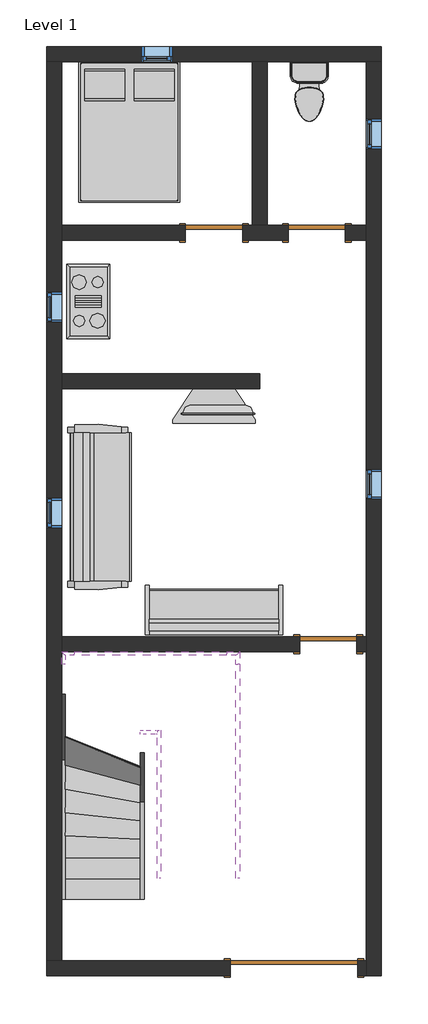
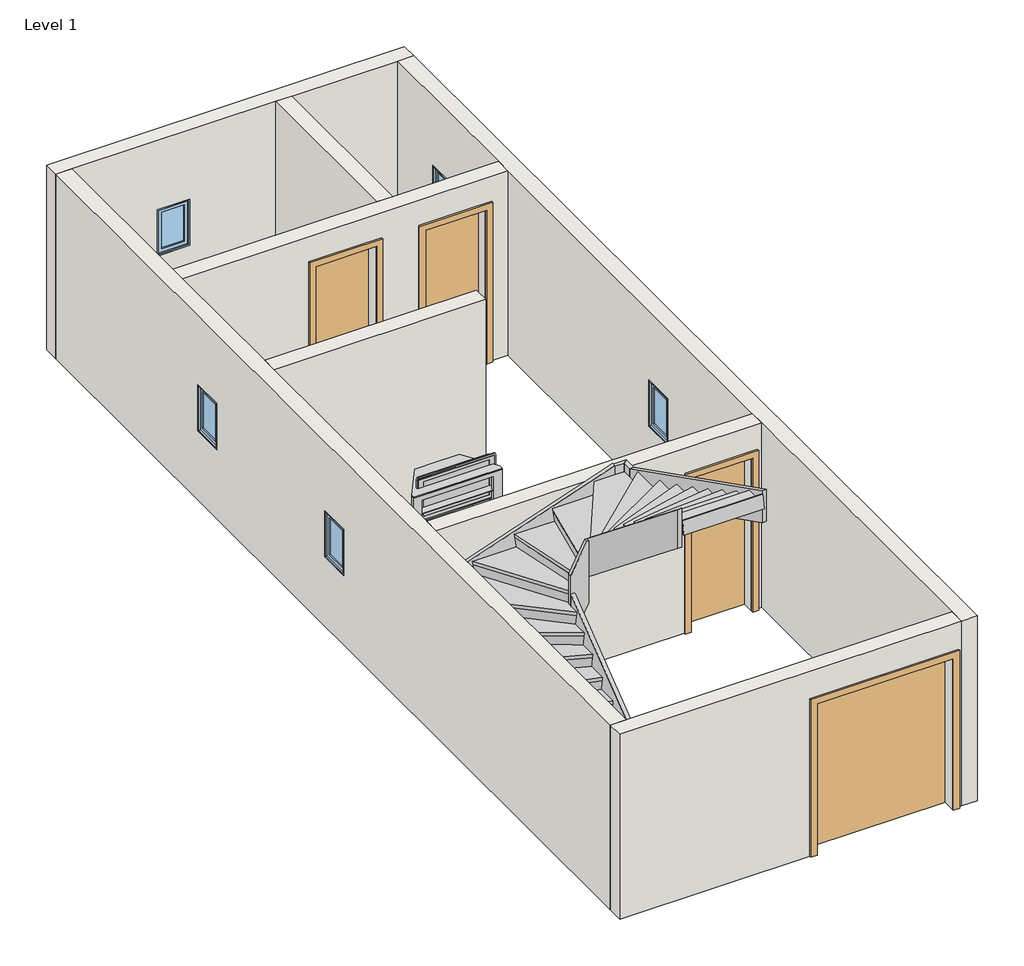
# One storey, incomplete: 10 members, 8 walls, 5 furniture elements, 5 windows, 4 doors, 1 flow terminal, 1 proxy, 1 stair flight.
"""IFC4 building model written with IfcOpenShell, lengths in millimetres."""

from ifc_helpers import new_model, si_unit, frame, origin, origin_with_axes, place, context, project, spatial, polyline, outline, extrude, faceted_brep, transform, mapped, element, save
from components import m_cook_top_4_unit_0915_x_500mm_0d6b06ed, m_door_double_flush_panel_double_acting_1700_x_2000mm_0a6d9c7f, m_single_flush_0762_x_2032mm_0c256fab, m_toilet_domestic_3d_m_toilet_domestic_3d_5cb52bd4, m_toilet_domestic_3d_m_toilet_domestic_3d_183bbd19, furniture_40ec15d9, furniture_0940mm_4831bac8, m_bed_box_1346_x_1880mm_double_b32eb57e, m_sofa_1830mm_f9e8a66b, m_sofa_pensi_2134mm_91f3548c, stair_flight_50mm_tread_25mm_nosing_13mm_riser_90fcb94b, m_fixed_0406_x_0610mm_8205b201

model = new_model("IFC4")

# Units and contexts
model_context = context("Model", 3, world=origin())
ifc_project = project(units=[si_unit("LENGTHUNIT", "METRE", prefix="MILLI")], contexts=[model_context])

# Site, building, storey
site = spatial("IfcSite", under=ifc_project)
building = spatial("IfcBuilding", under=site)
storey = spatial("IfcBuildingStorey", under=building, Name="Level 1", Elevation=0.0)

# Proxy
placement = place(None, origin())
m_cook_top_4_unit_0915_x_500mm_shape = m_cook_top_4_unit_0915_x_500mm_0d6b06ed(model_context)
element("IfcBuildingElementProxy", 1, Name="M_Cook Top-4 Unit : 0915 x 500mm", ObjectType="M_Cook Top-4 Unit : 0915 x 500mm", at=placement, inside=storey, context=model_context, shape_type="MappedRepresentation", body=[
    mapped(m_cook_top_4_unit_0915_x_500mm_shape, transform((-8350.9652156, 7282.492595, 0.0), x_axis=(0.0, 1.0000000000000002, 0.0), y_axis=(-1.0000000000000002, 0.0, 0.0), z_axis=(0.0, 0.0, 1.0))),
])

# Doors
m_door_double_flush_panel_double_acting_1700_x_2000mm_shape = m_door_double_flush_panel_double_acting_1700_x_2000mm_0a6d9c7f(model_context)
element("IfcDoor", 2, ObjectType="M_Door-Double-Flush_Panel-Double-Acting : 1700 x 2000mm", at=placement, inside=storey, context=model_context, shape_type="MappedRepresentation", body=[
    mapped(m_door_double_flush_panel_double_acting_1700_x_2000mm_shape, transform((-5607.7652156, -1609.107405, 0.0), x_axis=(1.0, 0.0, 0.0), y_axis=(0.0, 1.0, 0.0), z_axis=(0.0, 0.0, 1.0))),
])
m_single_flush_0762_x_2032mm_shape = m_single_flush_0762_x_2032mm_0c256fab(model_context)
element("IfcDoor", 3, ObjectType="M_Single-Flush : 0762 x 2032mm", at=placement, inside=storey, context=model_context, shape_type="MappedRepresentation", body=[
    mapped(m_single_flush_0762_x_2032mm_shape, transform((-6674.5652156, 8196.892595, 0.0), x_axis=(1.0, 0.0, 0.0), y_axis=(0.0, 1.0, 0.0), z_axis=(0.0, 0.0, 1.0))),
])
element("IfcDoor", 4, ObjectType="M_Single-Flush : 0762 x 2032mm", at=placement, inside=storey, context=model_context, shape_type="MappedRepresentation", body=[
    mapped(m_single_flush_0762_x_2032mm_shape, transform((-5302.9652156, 8196.892595, 0.0), x_axis=(1.0, 0.0, 0.0), y_axis=(0.0, 1.0, 0.0), z_axis=(0.0, 0.0, 1.0))),
])
element("IfcDoor", 5, ObjectType="M_Single-Flush : 0762 x 2032mm", at=placement, inside=storey, context=model_context, shape_type="MappedRepresentation", body=[
    mapped(m_single_flush_0762_x_2032mm_shape, transform((-5150.5652156, 2710.492595, 0.0), x_axis=(1.0, 0.0, 0.0), y_axis=(0.0, 1.0, 0.0), z_axis=(0.0, 0.0, 1.0))),
])

# Flow terminal
m_toilet_domestic_3d_m_toilet_domestic_3d_shape = m_toilet_domestic_3d_m_toilet_domestic_3d_5cb52bd4(model_context)
m_toilet_domestic_3d_m_toilet_domestic_3d_2_shape = m_toilet_domestic_3d_m_toilet_domestic_3d_183bbd19(model_context)
element("IfcFlowTerminal", 6, ObjectType="M_Toilet-Domestic-3D : M_Toilet-Domestic-3D", at=placement, inside=storey, context=model_context, shape_type="MappedRepresentation", body=[
    mapped(m_toilet_domestic_3d_m_toilet_domestic_3d_shape, transform((-5403.961243, 9988.1965677, 0.0), x_axis=(1.0, 0.0, 0.0), y_axis=(0.0, 1.0, 0.0), z_axis=(0.0, 0.0, 1.0))),
    mapped(m_toilet_domestic_3d_m_toilet_domestic_3d_2_shape, transform((-5403.961243, 9988.1965677, 0.0), x_axis=(1.0, 0.0, 0.0), y_axis=(0.0, 1.0, 0.0), z_axis=(0.0, 0.0, 1.0))),
])

# Furniture
furniture_shape = furniture_40ec15d9(model_context)
element("IfcFurniture", 7, at=placement, inside=storey, context=model_context, shape_type="MappedRepresentation", body=[
    mapped(furniture_shape, transform((-6799.7532177, 6115.692595, 0.0), x_axis=(1.0, 0.0, 0.0), y_axis=(0.0, 1.0, 0.0), z_axis=(0.0, 0.0, 1.0))),
])
furniture_0940mm_shape = furniture_0940mm_4831bac8(model_context)
element("IfcFurniture", 8, ObjectType="0940mm", at=placement, inside=storey, context=model_context, shape_type="MappedRepresentation", body=[
    mapped(furniture_0940mm_shape, transform((-6619.8207015, 5844.2185016, 0.0), x_axis=(1.0, 0.0, 0.0), y_axis=(0.0, 1.0, 0.0), z_axis=(0.0, 0.0, 1.0))),
])
m_bed_box_1346_x_1880mm_double_shape = m_bed_box_1346_x_1880mm_double_b32eb57e(model_context)
element("IfcFurniture", 9, ObjectType="M_Bed-Box : 1346 x 1880mm - Double", at=placement, inside=storey, context=model_context, shape_type="MappedRepresentation", body=[
    mapped(m_bed_box_1346_x_1880mm_double_shape, transform((-8143.9176746, 9777.3221032, 0.0), x_axis=(1.0, 0.0, 0.0), y_axis=(0.0, 1.0, 0.0), z_axis=(0.0, 0.0, 1.0))),
])
m_sofa_1830mm_shape = m_sofa_1830mm_f9e8a66b(model_context)
element("IfcFurniture", 10, ObjectType="M_Sofa : 1830mm", at=placement, inside=storey, context=model_context, shape_type="MappedRepresentation", body=[
    mapped(m_sofa_1830mm_shape, transform((-6604.1947238, 3313.8466934, 0.0), x_axis=(-1.0000000000000004, 0.0, 0.0), y_axis=(0.0, -1.0000000000000004, 0.0), z_axis=(0.0, 0.0, 1.0))),
])
m_sofa_pensi_2134mm_shape = m_sofa_pensi_2134mm_91f3548c(model_context)
element("IfcFurniture", 11, ObjectType="M_Sofa-Pensi : 2134mm", at=placement, inside=storey, context=model_context, shape_type="MappedRepresentation", body=[
    mapped(m_sofa_pensi_2134mm_shape, transform((-7921.4553795, 4260.686345, 0.0), x_axis=(0.0, 1.0, 0.0), y_axis=(-1.0, 0.0, 0.0), z_axis=(0.0, 0.0, 1.0))),
])

# Members
element("IfcMember", 12, ObjectType="Stringer - 50mm Width", at=placement, inside=storey, context=model_context, shape_type="SweptSolid", body=[
    extrude(outline(polyline([(-689.3306191, 0.0), (-689.3306191, 237.7763786), (2445.6423401, 1858.1790604), (2445.6423401, 1407.9055029), (-278.2149643, 0.0), (-689.3306191, 0.0)])), frame((-8708.1652156, 0.0, 0.0), z_axis=(1.0, 0.0, 0.0), x_axis=(0.0, 1.0, 0.0)), (0.0, 0.0, 1.0), 50.0),
])
element("IfcMember", 13, ObjectType="Stringer - 50mm Width", at=placement, inside=storey, context=model_context, shape_type="SweptSolid", body=[
    extrude(outline(polyline([(-8658.1652156, 2445.6423401), (-8708.1652156, 2445.6423401), (-8708.1652156, 2610.492595), (-8658.1652156, 2560.492595), (-8658.1652156, 2445.6423401)])), frame((0.0, 0.0, 1407.9055029), z_axis=(0.0, 0.0, 1.0), x_axis=(1.0, 0.0, 0.0)), (0.0, 0.0, 1.0), 450.2735574),
])
element("IfcMember", 14, ObjectType="Stringer - 50mm Width", at=placement, inside=storey, context=model_context, shape_type="SweptSolid", body=[
    extrude(outline(polyline([(-8658.1652156, 2560.492595), (-8708.1652156, 2610.492595), (-8536.9547066, 2610.492595), (-8536.9547066, 2560.492595), (-8658.1652156, 2560.492595)])), frame((0.0, 0.0, 1407.9055029), z_axis=(0.0, 0.0, 1.0), x_axis=(1.0, 0.0, 0.0)), (0.0, 0.0, 1.0), 450.2735574),
])
element("IfcMember", 15, ObjectType="Stringer - 50mm Width", at=placement, inside=storey, context=model_context, shape_type="SweptSolid", body=[
    extrude(outline(polyline([(1858.1790604, -8536.9547066), (1407.9055029, -8536.9547066), (2103.5576768, -6502.8954819), (2553.8312343, -6502.8954819), (1858.1790604, -8536.9547066)])), frame((0.0, 2560.492595, 0.0), z_axis=(0.0, 1.0, 0.0), x_axis=(0.0, 0.0, 1.0)), (0.0, 0.0, 1.0), 50.0),
])
element("IfcMember", 16, ObjectType="Stringer - 50mm Width", at=placement, inside=storey, context=model_context, shape_type="SweptSolid", body=[
    extrude(outline(polyline([(-6502.8954819, 2560.492595), (-6502.8954819, 2610.492595), (-6333.1136531, 2610.492595), (-6383.1136531, 2560.492595), (-6502.8954819, 2560.492595)])), frame((0.0, 0.0, 2121.8553305), z_axis=(0.0, 0.0, 1.0), x_axis=(1.0, 0.0, 0.0)), (0.0, 0.0, 1.0), 422.7463197),
])
element("IfcMember", 17, ObjectType="Stringer - 50mm Width", at=placement, inside=storey, context=model_context, shape_type="SweptSolid", body=[
    extrude(outline(polyline([(-6383.1136531, 2560.492595), (-6333.1136531, 2610.492595), (-6333.1136531, 2442.5214684), (-6383.1136531, 2442.5214684), (-6383.1136531, 2560.492595)])), frame((0.0, 0.0, 2121.8553305), z_axis=(0.0, 0.0, 1.0), x_axis=(1.0, 0.0, 0.0)), (0.0, 0.0, 1.0), 422.7463197),
])
element("IfcMember", 18, ObjectType="Stringer - 50mm Width", at=placement, inside=storey, context=model_context, shape_type="SweptSolid", body=[
    extrude(outline(polyline([(2442.5214684, 2544.6016503), (2442.5214684, 2121.8553305), (-414.3306191, 3565.1327467), (-414.3306191, 3987.8790664), (2442.5214684, 2544.6016503)])), frame((-6383.1136531, 0.0, 0.0), z_axis=(1.0, 0.0, 0.0), x_axis=(0.0, 1.0, 0.0)), (0.0, 0.0, 1.0), 50.0),
])
element("IfcMember", 19, ObjectType="Stringer - 50mm Width", at=placement, inside=storey, context=model_context, shape_type="SweptSolid", body=[
    extrude(outline(polyline([(-689.3306191, 0.0), (-689.3306191, 189.4989591), (1510.4668138, 1898.4837123), (1510.4668138, 1391.9587893), (-281.2562345, 0.0), (-689.3306191, 0.0)])), frame((-7658.1394344, 0.0, 0.0), z_axis=(1.0, 0.0, 0.0), x_axis=(0.0, 1.0, 0.0)), (0.0, 0.0, 1.0), 50.0),
])
element("IfcMember", 20, ObjectType="Stringer - 50mm Width", at=placement, inside=storey, context=model_context, shape_type="SweptSolid", body=[
    extrude(outline(polyline([(2137.8523026, -7658.1394344), (1430.8029285, -7658.1394344), (1430.8029285, -7575.3363491), (1703.8772172, -7433.1394344), (2523.9527077, -7433.1394344), (2523.9527077, -7457.0868686), (2137.8523026, -7658.1394344)])), frame((0.0, 1510.4668138, 0.0), z_axis=(0.0, 1.0, 0.0), x_axis=(0.0, 0.0, 1.0)), (0.0, 0.0, 1.0), 50.0),
])
element("IfcMember", 21, ObjectType="Stringer - 50mm Width", at=placement, inside=storey, context=model_context, shape_type="SweptSolid", body=[
    extrude(outline(polyline([(1560.4668138, 2523.9527077), (1560.4668138, 2011.6830523), (-414.3306191, 3591.6768139), (-414.3306191, 4103.9464694), (1560.4668138, 2523.9527077)])), frame((-7433.1394344, 0.0, 0.0), z_axis=(1.0, 0.0, 0.0), x_axis=(0.0, 1.0, 0.0)), (0.0, 0.0, 1.0), 50.0),
])

# Stair flight
stair_flight_50mm_tread_25mm_nosing_13mm_riser_shape = stair_flight_50mm_tread_25mm_nosing_13mm_riser_90fcb94b(model_context)
element("IfcStairFlight", 22, ObjectType="50mm Tread 25mm Nosing 13mm Riser", at=placement, inside=storey, context=model_context, shape_type="MappedRepresentation", body=[
    mapped(stair_flight_50mm_tread_25mm_nosing_13mm_riser_shape, transform((0.0, 0.0, 0.0), x_axis=(1.0, 0.0, 0.0), y_axis=(0.0, 1.0, 0.0), z_axis=(0.0, 0.0, 1.0))),
])

# Walls
element("IfcWall", 23, ObjectType="Generic - 200mm", at=placement, inside=storey, context=model_context, shape_type="Brep", body=[
    faceted_brep([(-8908.1652156, 10482.892595, 0.0), (-8708.1652156, 10482.892595, 0.0), (-6164.9652156, 10482.892595, 0.0), (-5964.9652156, 10482.892595, 0.0), (-4640.9652156, 10482.892595, 0.0), (-4440.9652156, 10482.892595, 0.0), (-4440.9652156, 10482.892595, 2438.4), (-4640.9652156, 10482.892595, 2438.4), (-5964.9652156, 10482.892595, 2438.4), (-6164.9652156, 10482.892595, 2438.4), (-8708.1652156, 10482.892595, 2438.4), (-8908.1652156, 10482.892595, 2438.4), (-7233.5652156, 10482.892595, 915.0), (-7639.5652156, 10482.892595, 915.0), (-7639.5652156, 10482.892595, 1525.0), (-7233.5652156, 10482.892595, 1525.0), (-8908.1652156, 10682.892595, 0.0), (-8908.1652156, 10682.892595, 2438.4), (-4440.9652156, 10682.892595, 2438.4), (-4440.9652156, 10682.892595, 0.0), (-7233.5652156, 10682.892595, 915.0), (-7233.5652156, 10682.892595, 1525.0), (-7639.5652156, 10682.892595, 1525.0), (-7639.5652156, 10682.892595, 915.0)], [[[0, 1, 2, 3, 4, 5, 6, 7, 8, 9, 10, 11], [12, 13, 14, 15]], [[16, 17, 18, 19], [20, 21, 22, 23]], [[5, 4, 3, 2, 1, 0, 16, 19]], [[11, 10, 9, 8, 7, 6, 18, 17]], [[6, 5, 19, 18]], [[0, 11, 17, 16]], [[21, 20, 12, 15]], [[22, 21, 15, 14]], [[23, 22, 14, 13]], [[20, 23, 13, 12]]]),
])
element("IfcWall", 24, ObjectType="Generic - 200mm", at=placement, inside=storey, context=model_context, shape_type="Brep", body=[
    faceted_brep([(-4640.9652156, 10482.892595, 0.0), (-4640.9652156, 8296.892595, 0.0), (-4640.9652156, 8096.892595, 0.0), (-4640.9652156, 2810.492595, 0.0), (-4640.9652156, 2610.492595, 0.0), (-4640.9652156, -1509.107405, 0.0), (-4640.9652156, -1709.107405, 0.0), (-4640.9652156, -1709.107405, 2438.4), (-4640.9652156, -1509.107405, 2438.4), (-4640.9652156, 2610.492595, 2438.4), (-4640.9652156, 2810.492595, 2438.4), (-4640.9652156, 8096.892595, 2438.4), (-4640.9652156, 8296.892595, 2438.4), (-4640.9652156, 10482.892595, 2438.4), (-4640.9652156, 4641.092595, 915.0), (-4640.9652156, 5047.092595, 915.0), (-4640.9652156, 5047.092595, 1525.0), (-4640.9652156, 4641.092595, 1525.0), (-4640.9652156, 9313.092595, 915.0), (-4640.9652156, 9719.092595, 915.0), (-4640.9652156, 9719.092595, 1525.0), (-4640.9652156, 9313.092595, 1525.0), (-4440.9652156, 10482.892595, 0.0), (-4440.9652156, 10482.892595, 2438.4), (-4440.9652156, -1709.107405, 2438.4), (-4440.9652156, -1709.107405, 0.0), (-4440.9652156, 4641.092595, 915.0), (-4440.9652156, 4641.092595, 1525.0), (-4440.9652156, 5047.092595, 1525.0), (-4440.9652156, 5047.092595, 915.0), (-4440.9652156, 9313.092595, 915.0), (-4440.9652156, 9313.092595, 1525.0), (-4440.9652156, 9719.092595, 1525.0), (-4440.9652156, 9719.092595, 915.0)], [[[0, 1, 2, 3, 4, 5, 6, 7, 8, 9, 10, 11, 12, 13], [14, 15, 16, 17], [18, 19, 20, 21]], [[22, 23, 24, 25], [26, 27, 28, 29], [30, 31, 32, 33]], [[6, 5, 4, 3, 2, 1, 0, 22, 25]], [[13, 12, 11, 10, 9, 8, 7, 24, 23]], [[0, 13, 23, 22]], [[7, 6, 25, 24]], [[27, 26, 14, 17]], [[28, 27, 17, 16]], [[29, 28, 16, 15]], [[26, 29, 15, 14]], [[31, 30, 18, 21]], [[32, 31, 21, 20]], [[33, 32, 20, 19]], [[30, 33, 19, 18]]]),
])
element("IfcWall", 25, ObjectType="Generic - 200mm", at=placement, inside=storey, context=model_context, shape_type="Brep", body=[
    faceted_brep([(-8908.1652156, -1509.107405, 2438.4), (-8708.1652156, -1509.107405, 2438.4), (-4640.9652156, -1509.107405, 2438.4), (-4640.9652156, -1509.107405, 0.0), (-4757.7652156, -1509.107405, 0.0), (-4757.7652156, -1509.107405, 2000.0), (-6457.7652156, -1509.107405, 2000.0), (-6457.7652156, -1509.107405, 0.0), (-8708.1652156, -1509.107405, 0.0), (-8908.1652156, -1509.107405, 0.0), (-4640.9652156, -1709.107405, 2438.4), (-8908.1652156, -1709.107405, 2438.4), (-8908.1652156, -1709.107405, 0.0), (-6457.7652156, -1709.107405, 0.0), (-6457.7652156, -1709.107405, 2000.0), (-4757.7652156, -1709.107405, 2000.0), (-4757.7652156, -1709.107405, 0.0), (-4640.9652156, -1709.107405, 0.0)], [[[0, 1, 2, 3, 4, 5, 6, 7, 8, 9]], [[10, 11, 12, 13, 14, 15, 16, 17]], [[3, 17, 16, 4]], [[12, 9, 8, 7, 13]], [[2, 1, 0, 11, 10]], [[3, 2, 10, 17]], [[0, 9, 12, 11]], [[15, 5, 4, 16]], [[5, 15, 14, 6]], [[6, 14, 13, 7]]]),
])
element("IfcWall", 26, ObjectType="Generic - 200mm", at=placement, inside=storey, context=model_context, shape_type="Brep", body=[
    faceted_brep([(-8708.1652156, -1509.107405, 0.0), (-8708.1652156, 2610.492595, 0.0), (-8708.1652156, 2810.492595, 0.0), (-8708.1652156, 6115.692595, 0.0), (-8708.1652156, 6315.692595, 0.0), (-8708.1652156, 8096.892595, 0.0), (-8708.1652156, 8296.892595, 0.0), (-8708.1652156, 10482.892595, 0.0), (-8708.1652156, 10482.892595, 2438.4), (-8708.1652156, 8296.892595, 2438.4), (-8708.1652156, 8096.892595, 2438.4), (-8708.1652156, 6315.692595, 2438.4), (-8708.1652156, 6115.692595, 2438.4), (-8708.1652156, 2810.492595, 2438.4), (-8708.1652156, 2610.492595, 2438.4), (-8708.1652156, -1509.107405, 2438.4), (-8708.1652156, 7003.292595, 915.0), (-8708.1652156, 7003.292595, 1525.0), (-8708.1652156, 7409.292595, 1525.0), (-8708.1652156, 7409.292595, 915.0), (-8708.1652156, 4260.092595, 915.0), (-8708.1652156, 4260.092595, 1525.0), (-8708.1652156, 4666.092595, 1525.0), (-8708.1652156, 4666.092595, 915.0), (-8908.1652156, -1509.107405, 0.0), (-8908.1652156, -1509.107405, 2438.4), (-8908.1652156, 10482.892595, 2438.4), (-8908.1652156, 10482.892595, 0.0), (-8908.1652156, 7003.292595, 915.0), (-8908.1652156, 7409.292595, 915.0), (-8908.1652156, 7409.292595, 1525.0), (-8908.1652156, 7003.292595, 1525.0), (-8908.1652156, 4260.092595, 915.0), (-8908.1652156, 4666.092595, 915.0), (-8908.1652156, 4666.092595, 1525.0), (-8908.1652156, 4260.092595, 1525.0)], [[[0, 1, 2, 3, 4, 5, 6, 7, 8, 9, 10, 11, 12, 13, 14, 15], [16, 17, 18, 19], [20, 21, 22, 23]], [[24, 25, 26, 27], [28, 29, 30, 31], [32, 33, 34, 35]], [[7, 6, 5, 4, 3, 2, 1, 0, 24, 27]], [[15, 14, 13, 12, 11, 10, 9, 8, 26, 25]], [[8, 7, 27, 26]], [[0, 15, 25, 24]], [[17, 16, 28, 31]], [[18, 17, 31, 30]], [[19, 18, 30, 29]], [[16, 19, 29, 28]], [[21, 20, 32, 35]], [[22, 21, 35, 34]], [[23, 22, 34, 33]], [[20, 23, 33, 32]]]),
])
element("IfcWall", 27, ObjectType="Generic - 200mm", at=placement, inside=storey, context=model_context, shape_type="SweptSolid", body=[
    extrude(outline(polyline([(-6164.9652156, 8296.892595), (-6164.9652156, 10482.892595), (-5964.9652156, 10482.892595), (-5964.9652156, 8296.892595), (-6164.9652156, 8296.892595)])), origin_with_axes(), (0.0, 0.0, 1.0), 2438.4),
])
element("IfcWall", 28, ObjectType="Generic - 200mm", at=placement, inside=storey, context=model_context, shape_type="Brep", body=[
    faceted_brep([(-4921.9652156, 8096.892595, 2032.0), (-4921.9652156, 8096.892595, 0.0), (-4640.9652156, 8096.892595, 0.0), (-4640.9652156, 8096.892595, 2438.4), (-8708.1652156, 8096.892595, 2438.4), (-8708.1652156, 8096.892595, 0.0), (-7055.5652156, 8096.892595, 0.0), (-7055.5652156, 8096.892595, 2032.0), (-6293.5652156, 8096.892595, 2032.0), (-6293.5652156, 8096.892595, 0.0), (-5683.9652156, 8096.892595, 0.0), (-5683.9652156, 8096.892595, 2032.0), (-4640.9652156, 8296.892595, 0.0), (-4921.9652156, 8296.892595, 0.0), (-4921.9652156, 8296.892595, 2032.0), (-5683.9652156, 8296.892595, 2032.0), (-5683.9652156, 8296.892595, 0.0), (-5964.9652156, 8296.892595, 0.0), (-6164.9652156, 8296.892595, 0.0), (-6293.5652156, 8296.892595, 0.0), (-6293.5652156, 8296.892595, 2032.0), (-7055.5652156, 8296.892595, 2032.0), (-7055.5652156, 8296.892595, 0.0), (-8708.1652156, 8296.892595, 0.0), (-8708.1652156, 8296.892595, 2438.4), (-6164.9652156, 8296.892595, 2438.4), (-5964.9652156, 8296.892595, 2438.4), (-4640.9652156, 8296.892595, 2438.4)], [[[0, 1, 2, 3, 4, 5, 6, 7, 8, 9, 10, 11]], [[12, 13, 14, 15, 16, 17, 18, 19, 20, 21, 22, 23, 24, 25, 26, 27]], [[6, 5, 23, 22]], [[10, 9, 19, 18, 17, 16]], [[2, 1, 13, 12]], [[4, 3, 27, 26, 25, 24]], [[3, 2, 12, 27]], [[5, 4, 24, 23]], [[20, 19, 9, 8]], [[21, 20, 8, 7]], [[22, 21, 7, 6]], [[14, 13, 1, 0]], [[15, 14, 0, 11]], [[16, 15, 11, 10]]]),
])
element("IfcWall", 29, ObjectType="Generic - 200mm", at=placement, inside=storey, context=model_context, shape_type="SweptSolid", body=[
    extrude(outline(polyline([(-6064.9652156, 6115.692595), (-8708.1652156, 6115.692595), (-8708.1652156, 6315.692595), (-6064.9652156, 6315.692595), (-6064.9652156, 6115.692595)])), origin_with_axes(), (0.0, 0.0, 1.0), 2438.4),
])
element("IfcWall", 30, ObjectType="Generic - 200mm", at=placement, inside=storey, context=model_context, shape_type="SweptSolid", body=[
    extrude(outline(polyline([(2032.0, -4769.5652156), (0.0, -4769.5652156), (0.0, -4640.9652156), (2438.4, -4640.9652156), (2438.4, -8708.1652156), (0.0, -8708.1652156), (0.0, -5531.5652156), (2032.0, -5531.5652156), (2032.0, -4769.5652156)])), frame((0.0, 2610.492595, 0.0), z_axis=(0.0, 1.0, 0.0), x_axis=(0.0, 0.0, 1.0)), (0.0, 0.0, 1.0), 200.0),
])

# Windows
m_fixed_0406_x_0610mm_shape = m_fixed_0406_x_0610mm_8205b201(model_context)
element("IfcWindow", 31, ObjectType="M_Fixed : 0406 x 0610mm", at=placement, inside=storey, context=model_context, shape_type="MappedRepresentation", body=[
    mapped(m_fixed_0406_x_0610mm_shape, transform((-7436.5652156, 10595.892595, 0.0), x_axis=(-1.0, 0.0, 0.0), y_axis=(0.0, -1.0, 0.0), z_axis=(0.0, 0.0, 1.0))),
])
element("IfcWindow", 32, ObjectType="M_Fixed : 0406 x 0610mm", at=placement, inside=storey, context=model_context, shape_type="MappedRepresentation", body=[
    mapped(m_fixed_0406_x_0610mm_shape, transform((-8795.1652156, 7206.292595, 0.0), x_axis=(0.0, 1.0, 0.0), y_axis=(-1.0, 0.0, 0.0), z_axis=(0.0, 0.0, 1.0))),
])
element("IfcWindow", 33, ObjectType="M_Fixed : 0406 x 0610mm", at=placement, inside=storey, context=model_context, shape_type="MappedRepresentation", body=[
    mapped(m_fixed_0406_x_0610mm_shape, transform((-8795.1652156, 4463.092595, 0.0), x_axis=(0.0, 1.0, 0.0), y_axis=(-1.0, 0.0, 0.0), z_axis=(0.0, 0.0, 1.0))),
])
element("IfcWindow", 34, ObjectType="M_Fixed : 0406 x 0610mm", at=placement, inside=storey, context=model_context, shape_type="MappedRepresentation", body=[
    mapped(m_fixed_0406_x_0610mm_shape, transform((-4527.9652156, 4844.092595, 0.0), x_axis=(0.0, 1.0, 0.0), y_axis=(-1.0, 0.0, 0.0), z_axis=(0.0, 0.0, 1.0))),
])
element("IfcWindow", 35, ObjectType="M_Fixed : 0406 x 0610mm", at=placement, inside=storey, context=model_context, shape_type="MappedRepresentation", body=[
    mapped(m_fixed_0406_x_0610mm_shape, transform((-4527.9652156, 9516.092595, 0.0), x_axis=(0.0, 1.0, 0.0), y_axis=(-1.0, 0.0, 0.0), z_axis=(0.0, 0.0, 1.0))),
])

save(model, "model.ifc")

# Revit data of these elements
# Type "M_Cook Top-4 Unit : 0915 x 500mm"
#   Counter Height = 900 mm
#   Depth = 500 mm
#   Width = 915 mm
#   Burner Material = Steel, Chrome Plated
#   Cooktop Material = Steel, Polished
#   Default Elevation = 0
# Type "M_Door-Double-Flush_Panel-Double-Acting : 1700 x 2000mm"
#   Type Mark = "22"
#   Construction Type Id = "DOOR"
#   Assembly Code = "C1020"
#   Analytic Construction = "Wooden"
#   W = 850 mm
#   Thickness = 50 mm
#   Thermal Resistance (R) = 0.455703 (m²·K)/W
#   Swing Angle [instance default] = 90.00°
#   Heat Transfer Coefficient (U) = 2.19465 W/(m²·K)
#   Height = 2000 mm
#   Trim Projection Ext. = 25 mm
#   Trim Projection Int. = 25 mm
#   Trim Width Ext. = 80 mm
#   Trim Width Int. = 80 mm
#   Width = 1700 mm
#   Define Thermal Properties by = 1
#   Panel Material = Wood - Birch - Solid Stained Light Low Gloss
#   Trim Material = Paint - Sienna
#   Visual Light Transmittance = 0
#   Solar Heat Gain Coefficient = 0
#   Function = (empty or 0)
#   Wall Closure = (empty or 0)
# Type "M_Single-Flush : 0762 x 2032mm"
#   Type Mark = "19"
#   Thickness = 51 mm
#   Height = 2032 mm
#   Trim Projection Ext = 25 mm
#   Trim Projection Int = 25 mm
#   Trim Width = 76 mm
#   Width = 762 mm
#   Door Material = Door - Panel
#   Frame Material = Door - Frame
#   Function = (empty or 0)
#   Wall Closure = (empty or 0)
# Type "M_Toilet-Domestic-3D : M_Toilet-Domestic-3D"
#   Bowl/Basin Material = Porcelain, Linen
#   Seat Material = Laminate, Linen, Matte
#   Default Elevation = 0
# Type
#   Depth = 460 mm
#   Width = 1100 mm
#   Height = 500 mm
#   Finish = Melamine - Gray
#   Default Elevation = 0
# Type "0940mm"
#   SinAng = 0.49 mm
#   L = 819.263 mm
#   H = 460.878 mm
#   Thickness = 110 mm
#   Diagonal = 940 mm
#   CosAng = 0.872 mm
#   Stand [instance default] = yes
#   Default Elevation = 0
# Type "M_Bed-Box : 1346 x 1880mm - Double"
#   Length = 1880 mm
#   Width = 1346 mm
#   Frame Material = Birch
#   Mattress Material = Linen, White
#   Default Elevation = 0
# Type "M_Sofa : 1830mm"
#   Width = 1830 mm
#   Seat Material = Linen, Beige
#   Frame Material = Cherry
#   Default Elevation = 0
# Type "M_Sofa-Pensi : 2134mm"
#   Length = 2134 mm
#   Sofa Material = Linen, Beige
#   Frame Material = Steel, Chrome Plated
#   Default Elevation = 0
# Type "Generic - 200mm"
#   Layers, outside or top first: 200 mm no material (function 1)
# Type "M_Fixed : 0406 x 0610mm"
#   Type Mark = "10"
#   Height = 610 mm
#   Default Sill Height = 915 mm
#   Width = 406 mm
#   Window Inset = 19 mm
#   Frame Exterior Material = Sash
#   Frame Interior Material = Sash
#   Glass Pane Material = Glass
#   Sash = Sash
#   Wall Closure = (empty or 0)
# Element 1 (IfcBuildingElementProxy, "M_Cook Top-4 Unit : 0915 x 500mm")
#   Phase Created = New Construction
#   Materials on its faces: "Steel, Chrome Plated", "Steel, Polished"
# Element 2 (IfcDoor, "M_Door-Double-Flush_Panel-Double-Acting : 1700 x 2000mm")
#   Swing Angle = 90.00°
#   Phase Created = New Construction
#   Materials on its faces: "Paint - Sienna", "Wood - Birch - Solid Stained Light Low Gloss"
# Elements 3, 4, 5 (IfcDoor, "M_Single-Flush : 0762 x 2032mm")
#   Phase Created = New Construction
#   Materials on its faces: "Door - Frame", "Door - Panel"
# Element 6 (IfcFlowTerminal, "M_Toilet-Domestic-3D : M_Toilet-Domestic-3D")
#   Mark = "1"
#   Phase Created = New Construction
#   Materials on its faces: "Porcelain, Linen", "Laminate, Linen, Matte"
# Element 7 (IfcFurniture)
#   Phase Created = New Construction
#   Materials on its faces: "Melamine - Gray", "Glass - Shelves"
# Element 8 (IfcFurniture, "0940mm")
#   Stand = yes
#   Phase Created = New Construction
#   Materials on its faces: "TV - Black", "TV - Glass", "TV - Screen"
# Element 9 (IfcFurniture, "M_Bed-Box : 1346 x 1880mm - Double")
#   Phase Created = New Construction
#   Materials on its faces: "Birch", "Linen, White"
# Element 10 (IfcFurniture, "M_Sofa : 1830mm")
#   Phase Created = New Construction
#   Materials on its faces: "Cherry", "Linen, Beige"
# Element 11 (IfcFurniture, "M_Sofa-Pensi : 2134mm")
#   Phase Created = New Construction
#   Materials on its faces: "Linen, Beige", "Steel, Chrome Plated"
# Elements 12, 13, 14, 15, 16, 17, 18, 19, 20, 21 (IfcMember, "Stringer - 50mm Width")
#   Phase Created = New Construction
# Element 22 (IfcStairFlight, "50mm Tread 25mm Nosing 13mm Riser")
#   Phase Created = New Construction
# Elements 23, 24, 25, 26, 27, 28, 29, 30 (IfcWall, "Generic - 200mm")
#   Top Offset = 0 mm
#   Base Offset = 0 mm
#   Unconnected Height = 2438.4 mm
#   wall height = 2438.4 mm
#   Phase Created = New Construction
#   Base Constraint = Level 1
#   Materials on its faces: "Default Wall"
# Element 31 (IfcWindow, "M_Fixed : 0406 x 0610mm")
#   Mark = "6"
#   Phase Created = New Construction
#   Materials on its faces: "Sash", "Glass"
# Element 32 (IfcWindow, "M_Fixed : 0406 x 0610mm")
#   Mark = "7"
#   Phase Created = New Construction
#   Materials on its faces: "Sash", "Glass"
# Element 33 (IfcWindow, "M_Fixed : 0406 x 0610mm")
#   Mark = "8"
#   Phase Created = New Construction
#   Materials on its faces: "Sash", "Glass"
# Element 34 (IfcWindow, "M_Fixed : 0406 x 0610mm")
#   Mark = "9"
#   Phase Created = New Construction
#   Materials on its faces: "Sash", "Glass"
# Element 35 (IfcWindow, "M_Fixed : 0406 x 0610mm")
#   Mark = "10"
#   Phase Created = New Construction
#   Materials on its faces: "Sash", "Glass"
# Materials
#   "Steel, Chrome Plated": class "Metal", colour RGB 244 244 244, transparency 0, Description = "Chromiuim plated steel", Cost = 0
#   "Steel, Polished": class "Metal", colour RGB 57 57 57, transparency 0, Description = "Polished steel", Cost = 0
#   "Wood - Birch - Solid Stained Light Low Gloss": class "Wood", colour RGB 210 159 95, transparency 0, Cost = 0
#   "Paint - Sienna": colour RGB 118 70 51, transparency 0, Cost = 0
#   "Door - Panel": class "Wood", colour RGB 114 82 51, transparency 0
#   "Door - Frame": colour RGB 153 76 43, transparency 0
#   "Porcelain, Linen": class "Ceramic", colour RGB 249 239 230, transparency 0, Description = "Porcelain, linen", Cost = 0
#   "Laminate, Linen, Matte": class "Plastic", colour RGB 249 239 230, transparency 0, Description = "Plastic Laminate - Linen, Matte", Cost = 0
#   "Melamine - Gray": class "Wood", colour RGB 49 49 49, transparency 0
#   "Birch": class "Wood", colour RGB 224 178 126, transparency 0, Description = "Betula Alleghaniensis", Cost = 0
#   "Linen, White": class "Textile", colour RGB 247 247 239, transparency 0, Description = "Linen, white", Cost = 0
#   "Linen, Beige": class "Textile", colour RGB 249 239 230, transparency 0, Description = "Linen, beige", Cost = 0
#   "Cherry": class "Wood", colour RGB 154 107 61, transparency 0, Description = "Prunus Serotina", Cost = 0
#   "Sash": class "Wood", colour RGB 136 99 55, transparency 0
#   "Glass": class "Glass", colour RGB 218 227 224, transparency 0.85, Description = "Soda Lime Glass", Cost = 0
#   "Glass - Shelves": class "Glass", colour RGB 167 167 167, transparency 0.9
#   "TV - Black": colour RGB 49 49 49, transparency 0
#   "TV - Glass": colour RGB 157 157 157, transparency 0.9
#   "TV - Screen": colour RGB 0 0 0, transparency 0
#   "Default Wall": colour RGB 80 80 80, transparency 0
